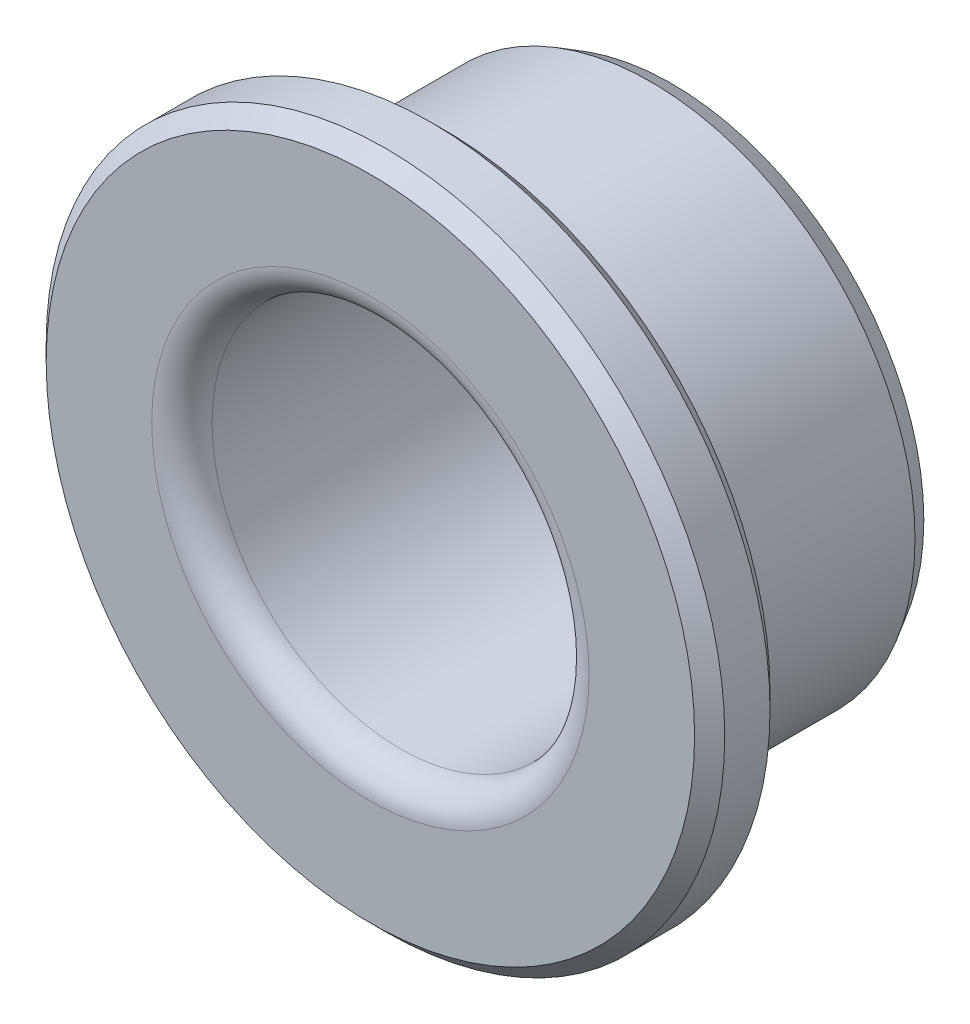
ISO-10303-21;
HEADER;
FILE_DESCRIPTION(('STEP AP214'),'2;1');
FILE_NAME('part.step','',(''),(''),'','','');
FILE_SCHEMA(('AUTOMOTIVE_DESIGN { 1 0 10303 214 1 1 1 1 }'));
ENDSEC;
DATA;
#1=APPLICATION_CONTEXT('core data for automotive mechanical design processes');
#2=APPLICATION_PROTOCOL_DEFINITION('international standard','automotive_design',2000,#1);
#3=PRODUCT_CONTEXT('',#1,'mechanical');
#4=PRODUCT('Part','Part','',(#3));
#5=PRODUCT_RELATED_PRODUCT_CATEGORY('part','',(#4));
#6=PRODUCT_DEFINITION_FORMATION('','',#4);
#7=PRODUCT_DEFINITION_CONTEXT('part definition',#1,'design');
#8=PRODUCT_DEFINITION('design','',#6,#7);
#9=PRODUCT_DEFINITION_SHAPE('','',#8);
#10=(LENGTH_UNIT() NAMED_UNIT(*) SI_UNIT(.MILLI.,.METRE.));
#11=(NAMED_UNIT(*) PLANE_ANGLE_UNIT() SI_UNIT($,.RADIAN.));
#12=(NAMED_UNIT(*) SI_UNIT($,.STERADIAN.) SOLID_ANGLE_UNIT());
#13=UNCERTAINTY_MEASURE_WITH_UNIT(LENGTH_MEASURE(1.E-05),#10,'distance_accuracy_value','');
#14=(GEOMETRIC_REPRESENTATION_CONTEXT(3) GLOBAL_UNCERTAINTY_ASSIGNED_CONTEXT((#13)) GLOBAL_UNIT_ASSIGNED_CONTEXT((#10,
#11,#12)) REPRESENTATION_CONTEXT('',''));
#15=CARTESIAN_POINT('',(0.,0.,0.));
#16=DIRECTION('',(0.,0.,1.));
#17=DIRECTION('',(1.,0.,0.));
#18=AXIS2_PLACEMENT_3D('',#15,#16,#17);
#19=CARTESIAN_POINT('',(0.,0.,15.));
#20=DIRECTION('',(0.,0.,-1.));
#21=DIRECTION('',(-1.,0.,0.));
#22=AXIS2_PLACEMENT_3D('',#19,#20,#21);
#23=CYLINDRICAL_SURFACE('',#22,17.5);
#24=CARTESIAN_POINT('',(0.,0.,1.38564064605511));
#25=DIRECTION('',(0.,0.,1.));
#26=DIRECTION('',(1.,0.,0.));
#27=AXIS2_PLACEMENT_3D('',#24,#25,#26);
#28=CIRCLE('',#27,17.5);
#29=CARTESIAN_POINT('',(17.5,0.,1.38564064605511));
#30=VERTEX_POINT('',#29);
#31=EDGE_CURVE('E77',#30,#30,#28,.T.);
#32=ORIENTED_EDGE('',*,*,#31,.T.);
#33=EDGE_LOOP('',(#32));
#34=FACE_BOUND('',#33,.T.);
#35=CARTESIAN_POINT('',(0.,0.,15.));
#36=DIRECTION('',(0.,0.,1.));
#37=DIRECTION('',(1.,0.,0.));
#38=AXIS2_PLACEMENT_3D('',#35,#36,#37);
#39=CIRCLE('',#38,17.5);
#40=CARTESIAN_POINT('',(17.5,0.,15.));
#41=VERTEX_POINT('',#40);
#42=EDGE_CURVE('E79',#41,#41,#39,.T.);
#43=ORIENTED_EDGE('',*,*,#42,.F.);
#44=EDGE_LOOP('',(#43));
#45=FACE_BOUND('',#44,.T.);
#46=ADVANCED_FACE('F41',(#34,#45),#23,.T.);
#47=CARTESIAN_POINT('',(0.,0.,0.));
#48=DIRECTION('',(0.,0.,1.));
#49=DIRECTION('',(1.,0.,0.));
#50=AXIS2_PLACEMENT_3D('',#47,#48,#49);
#51=PLANE('',#50);
#52=CARTESIAN_POINT('',(0.,0.,0.));
#53=DIRECTION('',(0.,0.,1.));
#54=DIRECTION('',(1.,0.,0.));
#55=AXIS2_PLACEMENT_3D('',#52,#53,#54);
#56=CIRCLE('',#55,13.5);
#57=CARTESIAN_POINT('',(13.5,0.,0.));
#58=VERTEX_POINT('',#57);
#59=EDGE_CURVE('E48',#58,#58,#56,.T.);
#60=ORIENTED_EDGE('',*,*,#59,.T.);
#61=EDGE_LOOP('',(#60));
#62=FACE_BOUND('',#61,.T.);
#63=CARTESIAN_POINT('',(0.,0.,0.));
#64=DIRECTION('',(0.,0.,1.));
#65=DIRECTION('',(1.,0.,0.));
#66=AXIS2_PLACEMENT_3D('',#63,#64,#65);
#67=CIRCLE('',#66,16.7);
#68=CARTESIAN_POINT('',(16.7,0.,0.));
#69=VERTEX_POINT('',#68);
#70=EDGE_CURVE('E73',#69,#69,#67,.F.);
#71=ORIENTED_EDGE('',*,*,#70,.T.);
#72=EDGE_LOOP('',(#71));
#73=FACE_BOUND('',#72,.T.);
#74=ADVANCED_FACE('F86',(#62,#73),#51,.F.);
#75=CARTESIAN_POINT('',(0.,0.,20.));
#76=DIRECTION('',(0.,0.,-1.));
#77=DIRECTION('',(-1.,0.,0.));
#78=AXIS2_PLACEMENT_3D('',#75,#76,#77);
#79=CYLINDRICAL_SURFACE('',#78,22.5);
#80=CARTESIAN_POINT('',(0.,0.,16.));
#81=DIRECTION('',(0.,0.,1.));
#82=DIRECTION('',(1.,0.,0.));
#83=AXIS2_PLACEMENT_3D('',#80,#81,#82);
#84=CIRCLE('',#83,22.5);
#85=CARTESIAN_POINT('',(22.5,0.,16.));
#86=VERTEX_POINT('',#85);
#87=EDGE_CURVE('E62',#86,#86,#84,.T.);
#88=ORIENTED_EDGE('',*,*,#87,.T.);
#89=EDGE_LOOP('',(#88));
#90=FACE_BOUND('',#89,.T.);
#91=CARTESIAN_POINT('',(0.,0.,19.));
#92=DIRECTION('',(0.,0.,1.));
#93=DIRECTION('',(1.,0.,0.));
#94=AXIS2_PLACEMENT_3D('',#91,#92,#93);
#95=CIRCLE('',#94,22.5);
#96=CARTESIAN_POINT('',(22.5,0.,19.));
#97=VERTEX_POINT('',#96);
#98=EDGE_CURVE('E61',#97,#97,#95,.F.);
#99=ORIENTED_EDGE('',*,*,#98,.T.);
#100=EDGE_LOOP('',(#99));
#101=FACE_BOUND('',#100,.T.);
#102=ADVANCED_FACE('F93',(#90,#101),#79,.T.);
#103=CARTESIAN_POINT('',(0.,0.,20.));
#104=DIRECTION('',(0.,0.,1.));
#105=DIRECTION('',(1.,0.,0.));
#106=AXIS2_PLACEMENT_3D('',#103,#104,#105);
#107=PLANE('',#106);
#108=CARTESIAN_POINT('',(0.,0.,20.));
#109=DIRECTION('',(0.,0.,1.));
#110=DIRECTION('',(1.,0.,0.));
#111=AXIS2_PLACEMENT_3D('',#108,#109,#110);
#112=CIRCLE('',#111,21.5);
#113=CARTESIAN_POINT('',(21.5,0.,20.));
#114=VERTEX_POINT('',#113);
#115=EDGE_CURVE('E55',#114,#114,#112,.T.);
#116=ORIENTED_EDGE('',*,*,#115,.T.);
#117=EDGE_LOOP('',(#116));
#118=FACE_BOUND('',#117,.T.);
#119=CARTESIAN_POINT('',(0.,0.,20.));
#120=DIRECTION('',(0.,0.,1.));
#121=DIRECTION('',(1.,0.,0.));
#122=AXIS2_PLACEMENT_3D('',#119,#120,#121);
#123=CIRCLE('',#122,14.5);
#124=CARTESIAN_POINT('',(14.5,0.,20.));
#125=VERTEX_POINT('',#124);
#126=EDGE_CURVE('E70',#125,#125,#123,.F.);
#127=ORIENTED_EDGE('',*,*,#126,.T.);
#128=EDGE_LOOP('',(#127));
#129=FACE_BOUND('',#128,.T.);
#130=ADVANCED_FACE('F129',(#118,#129),#107,.T.);
#131=CARTESIAN_POINT('',(0.,0.,15.));
#132=DIRECTION('',(0.,0.,1.));
#133=DIRECTION('',(1.,0.,0.));
#134=AXIS2_PLACEMENT_3D('',#131,#132,#133);
#135=PLANE('',#134);
#136=CARTESIAN_POINT('',(0.,0.,15.));
#137=DIRECTION('',(0.,0.,1.));
#138=DIRECTION('',(1.,0.,0.));
#139=AXIS2_PLACEMENT_3D('',#136,#137,#138);
#140=CIRCLE('',#139,21.5);
#141=CARTESIAN_POINT('',(21.5,0.,15.));
#142=VERTEX_POINT('',#141);
#143=EDGE_CURVE('E57',#142,#142,#140,.F.);
#144=ORIENTED_EDGE('',*,*,#143,.T.);
#145=EDGE_LOOP('',(#144));
#146=FACE_BOUND('',#145,.T.);
#147=ORIENTED_EDGE('',*,*,#42,.T.);
#148=EDGE_LOOP('',(#147));
#149=FACE_BOUND('',#148,.T.);
#150=ADVANCED_FACE('F84',(#146,#149),#135,.F.);
#151=CARTESIAN_POINT('',(0.,0.,1.38564064605511));
#152=DIRECTION('',(0.,0.,1.));
#153=DIRECTION('',(1.,0.,0.));
#154=AXIS2_PLACEMENT_3D('',#151,#152,#153);
#155=CONICAL_SURFACE('',#154,17.5,0.523598775598298);
#156=CARTESIAN_POINT('',(16.7,0.,0.));
#157=CARTESIAN_POINT('',(16.7083333333333,0.,0.0144337567297409));
#158=CARTESIAN_POINT('',(16.7166666666667,0.,0.0288675134594815));
#159=CARTESIAN_POINT('',(16.7333333333333,0.,0.0577350269189626));
#160=CARTESIAN_POINT('',(16.7416666666667,0.,0.0721687836487032));
#161=CARTESIAN_POINT('',(16.7583333333333,0.,0.101036297108185));
#162=CARTESIAN_POINT('',(16.7666666666667,0.,0.115470053837926));
#163=CARTESIAN_POINT('',(16.7833333333333,0.,0.144337567297408));
#164=CARTESIAN_POINT('',(16.7916666666667,0.,0.158771324027148));
#165=CARTESIAN_POINT('',(16.8083333333333,0.,0.18763883748663));
#166=CARTESIAN_POINT('',(16.8166666666667,0.,0.20207259421637));
#167=CARTESIAN_POINT('',(16.8333333333333,0.,0.230940107675852));
#168=CARTESIAN_POINT('',(16.8416666666667,0.,0.245373864405593));
#169=CARTESIAN_POINT('',(16.8583333333333,0.,0.274241377865074));
#170=CARTESIAN_POINT('',(16.8666666666667,0.,0.288675134594815));
#171=CARTESIAN_POINT('',(16.8833333333333,0.,0.317542648054297));
#172=CARTESIAN_POINT('',(16.8916666666667,0.,0.331976404784037));
#173=CARTESIAN_POINT('',(16.9083333333333,0.,0.360843918243519));
#174=CARTESIAN_POINT('',(16.9166666666667,0.,0.375277674973259));
#175=CARTESIAN_POINT('',(16.9333333333333,0.,0.404145188432741));
#176=CARTESIAN_POINT('',(16.9416666666667,0.,0.418578945162482));
#177=CARTESIAN_POINT('',(16.9583333333333,0.,0.447446458621964));
#178=CARTESIAN_POINT('',(16.9666666666667,0.,0.461880215351704));
#179=CARTESIAN_POINT('',(16.9833333333333,0.,0.490747728811186));
#180=CARTESIAN_POINT('',(16.9916666666667,0.,0.505181485540926));
#181=CARTESIAN_POINT('',(17.0083333333333,0.,0.534048999000408));
#182=CARTESIAN_POINT('',(17.0166666666667,0.,0.548482755730149));
#183=CARTESIAN_POINT('',(17.0333333333333,0.,0.57735026918963));
#184=CARTESIAN_POINT('',(17.0416666666667,0.,0.591784025919371));
#185=CARTESIAN_POINT('',(17.0583333333333,0.,0.620651539378852));
#186=CARTESIAN_POINT('',(17.0666666666667,0.,0.635085296108593));
#187=CARTESIAN_POINT('',(17.0833333333333,0.,0.663952809568075));
#188=CARTESIAN_POINT('',(17.0916666666667,0.,0.678386566297816));
#189=CARTESIAN_POINT('',(17.1083333333333,0.,0.707254079757297));
#190=CARTESIAN_POINT('',(17.1166666666667,0.,0.721687836487038));
#191=CARTESIAN_POINT('',(17.1333333333333,0.,0.750555349946519));
#192=CARTESIAN_POINT('',(17.1416666666667,0.,0.76498910667626));
#193=CARTESIAN_POINT('',(17.1583333333333,0.,0.793856620135742));
#194=CARTESIAN_POINT('',(17.1666666666667,0.,0.808290376865482));
#195=CARTESIAN_POINT('',(17.1833333333333,0.,0.837157890324964));
#196=CARTESIAN_POINT('',(17.1916666666667,0.,0.851591647054704));
#197=CARTESIAN_POINT('',(17.2083333333333,0.,0.880459160514186));
#198=CARTESIAN_POINT('',(17.2166666666667,0.,0.894892917243927));
#199=CARTESIAN_POINT('',(17.2333333333333,0.,0.923760430703408));
#200=CARTESIAN_POINT('',(17.2416666666667,0.,0.938194187433149));
#201=CARTESIAN_POINT('',(17.2583333333333,0.,0.96706170089263));
#202=CARTESIAN_POINT('',(17.2666666666667,0.,0.981495457622371));
#203=CARTESIAN_POINT('',(17.2833333333333,0.,1.01036297108185));
#204=CARTESIAN_POINT('',(17.2916666666667,0.,1.02479672781159));
#205=CARTESIAN_POINT('',(17.3083333333333,0.,1.05366424127108));
#206=CARTESIAN_POINT('',(17.3166666666667,0.,1.06809799800082));
#207=CARTESIAN_POINT('',(17.3333333333333,0.,1.0969655114603));
#208=CARTESIAN_POINT('',(17.3416666666667,0.,1.11139926819004));
#209=CARTESIAN_POINT('',(17.3583333333333,0.,1.14026678164952));
#210=CARTESIAN_POINT('',(17.3666666666667,0.,1.15470053837926));
#211=CARTESIAN_POINT('',(17.3833333333333,0.,1.18356805183874));
#212=CARTESIAN_POINT('',(17.3916666666667,0.,1.19800180856848));
#213=CARTESIAN_POINT('',(17.4083333333333,0.,1.22686932202796));
#214=CARTESIAN_POINT('',(17.4166666666667,0.,1.24130307875771));
#215=CARTESIAN_POINT('',(17.4333333333333,0.,1.27017059221719));
#216=CARTESIAN_POINT('',(17.4416666666667,0.,1.28460434894693));
#217=CARTESIAN_POINT('',(17.4583333333333,0.,1.31347186240641));
#218=CARTESIAN_POINT('',(17.4666666666667,0.,1.32790561913615));
#219=CARTESIAN_POINT('',(17.4833333333333,0.,1.35677313259563));
#220=CARTESIAN_POINT('',(17.4916666666667,0.,1.37120688932537));
#221=CARTESIAN_POINT('',(17.5,0.,1.38564064605511));
#222=B_SPLINE_CURVE_WITH_KNOTS('',3,(#156,#157,#158,#159,#160,#161,#162,#163,#164,#165,#166,
#167,#168,#169,#170,#171,#172,#173,#174,#175,#176,#177,#178,#179,#180,#181,#182,#183,#184,#185,
#186,#187,#188,#189,#190,#191,#192,#193,#194,#195,#196,#197,#198,#199,#200,#201,#202,#203,#204,
#205,#206,#207,#208,#209,#210,#211,#212,#213,#214,#215,#216,#217,#218,#219,#220,#221),
.UNSPECIFIED.,.F.,.F.,(4,2,2,2,2,2,2,2,2,2,2,2,2,2,2,2,2,2,2,2,2,2,2,2,2,2,2,2,2,2,2,2,4),(0.,
0.0500000000000007,0.100000000000001,0.15,0.200000000000001,0.250000000000001,0.300000000000002,
0.350000000000003,0.400000000000003,0.450000000000004,0.500000000000003,0.550000000000004,
0.600000000000005,0.650000000000005,0.700000000000006,0.750000000000007,0.800000000000005,
0.850000000000006,0.900000000000007,0.950000000000008,1.00000000000001,1.05000000000001,
1.10000000000001,1.15000000000001,1.20000000000001,1.25000000000001,1.30000000000001,
1.35000000000001,1.40000000000001,1.45000000000001,1.50000000000001,1.55000000000001,
1.60000000000001),.UNSPECIFIED.);
#223=EDGE_CURVE('BSEAM96',#69,#30,#222,.T.);
#224=ORIENTED_EDGE('',*,*,#70,.F.);
#225=ORIENTED_EDGE('',*,*,#31,.F.);
#226=ORIENTED_EDGE('',*,*,#223,.T.);
#227=ORIENTED_EDGE('',*,*,#223,.F.);
#228=EDGE_LOOP('',(#224,#226,#225,#227));
#229=FACE_BOUND('',#228,.T.);
#230=ADVANCED_FACE('F96',(#229),#155,.T.);
#231=CARTESIAN_POINT('',(0.,0.,0.));
#232=DIRECTION('',(0.,0.,1.));
#233=DIRECTION('',(1.,0.,0.));
#234=AXIS2_PLACEMENT_3D('',#231,#232,#233);
#235=CYLINDRICAL_SURFACE('',#234,12.5);
#236=CARTESIAN_POINT('',(0.,0.,1.));
#237=DIRECTION('',(0.,0.,1.));
#238=DIRECTION('',(1.,0.,0.));
#239=AXIS2_PLACEMENT_3D('',#236,#237,#238);
#240=CIRCLE('',#239,12.5);
#241=CARTESIAN_POINT('',(12.5,0.,1.));
#242=VERTEX_POINT('',#241);
#243=EDGE_CURVE('E10',#242,#242,#240,.F.);
#244=ORIENTED_EDGE('',*,*,#243,.T.);
#245=EDGE_LOOP('',(#244));
#246=FACE_BOUND('',#245,.T.);
#247=CARTESIAN_POINT('',(0.,0.,18.));
#248=DIRECTION('',(0.,0.,1.));
#249=DIRECTION('',(1.,0.,0.));
#250=AXIS2_PLACEMENT_3D('',#247,#248,#249);
#251=CIRCLE('',#250,12.5);
#252=CARTESIAN_POINT('',(12.5,0.,18.));
#253=VERTEX_POINT('',#252);
#254=EDGE_CURVE('E69',#253,#253,#251,.T.);
#255=ORIENTED_EDGE('',*,*,#254,.T.);
#256=EDGE_LOOP('',(#255));
#257=FACE_BOUND('',#256,.T.);
#258=ADVANCED_FACE('F101',(#246,#257),#235,.F.);
#259=CARTESIAN_POINT('',(0.,0.,18.));
#260=DIRECTION('',(0.,0.,1.));
#261=DIRECTION('',(1.,0.,0.));
#262=AXIS2_PLACEMENT_3D('',#259,#260,#261);
#263=TOROIDAL_SURFACE('',#262,14.5,2.);
#264=ORIENTED_EDGE('',*,*,#126,.F.);
#265=EDGE_LOOP('',(#264));
#266=FACE_BOUND('',#265,.T.);
#267=ORIENTED_EDGE('',*,*,#254,.F.);
#268=EDGE_LOOP('',(#267));
#269=FACE_BOUND('',#268,.T.);
#270=ADVANCED_FACE('F102',(#266,#269),#263,.T.);
#271=CARTESIAN_POINT('',(0.,0.,16.));
#272=DIRECTION('',(0.,0.,1.));
#273=DIRECTION('',(1.,0.,0.));
#274=AXIS2_PLACEMENT_3D('',#271,#272,#273);
#275=CONICAL_SURFACE('',#274,22.5,0.78539816339745);
#276=ORIENTED_EDGE('',*,*,#143,.F.);
#277=EDGE_LOOP('',(#276));
#278=FACE_BOUND('',#277,.T.);
#279=ORIENTED_EDGE('',*,*,#87,.F.);
#280=EDGE_LOOP('',(#279));
#281=FACE_BOUND('',#280,.T.);
#282=ADVANCED_FACE('F108',(#278,#281),#275,.T.);
#283=CARTESIAN_POINT('',(0.,0.,20.));
#284=DIRECTION('',(0.,0.,-1.));
#285=DIRECTION('',(-1.,0.,0.));
#286=AXIS2_PLACEMENT_3D('',#283,#284,#285);
#287=CONICAL_SURFACE('',#286,21.5,0.785398163397452);
#288=ORIENTED_EDGE('',*,*,#98,.F.);
#289=EDGE_LOOP('',(#288));
#290=FACE_BOUND('',#289,.T.);
#291=ORIENTED_EDGE('',*,*,#115,.F.);
#292=EDGE_LOOP('',(#291));
#293=FACE_BOUND('',#292,.T.);
#294=ADVANCED_FACE('F112',(#290,#293),#287,.T.);
#295=CARTESIAN_POINT('',(0.,0.,1.));
#296=DIRECTION('',(0.,0.,1.));
#297=DIRECTION('',(1.,0.,0.));
#298=AXIS2_PLACEMENT_3D('',#295,#296,#297);
#299=TOROIDAL_SURFACE('',#298,13.5,1.);
#300=ORIENTED_EDGE('',*,*,#243,.F.);
#301=EDGE_LOOP('',(#300));
#302=FACE_BOUND('',#301,.T.);
#303=ORIENTED_EDGE('',*,*,#59,.F.);
#304=EDGE_LOOP('',(#303));
#305=FACE_BOUND('',#304,.T.);
#306=ADVANCED_FACE('F43',(#302,#305),#299,.T.);
#307=CLOSED_SHELL('',(#46,#74,#102,#130,#150,#230,#258,#270,#282,#294,#306));
#308=MANIFOLD_SOLID_BREP('B2',#307);
#309=ADVANCED_BREP_SHAPE_REPRESENTATION('',(#18,#308),#14);
#310=SHAPE_DEFINITION_REPRESENTATION(#9,#309);
ENDSEC;
END-ISO-10303-21;
